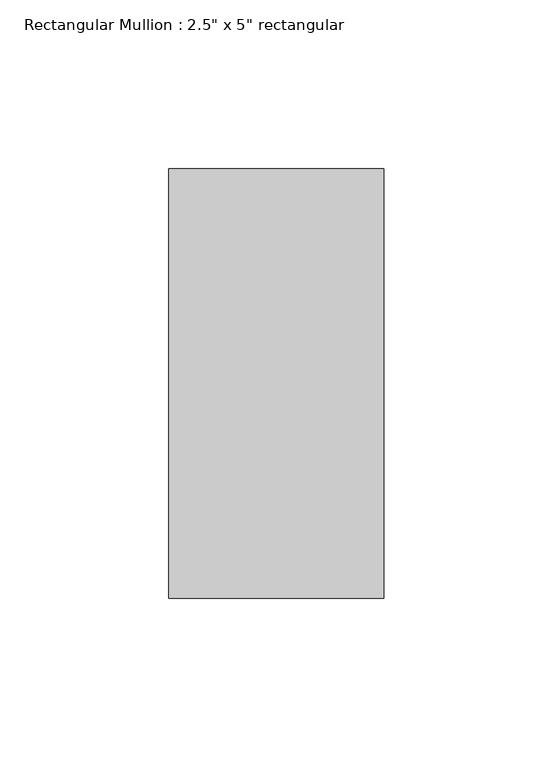
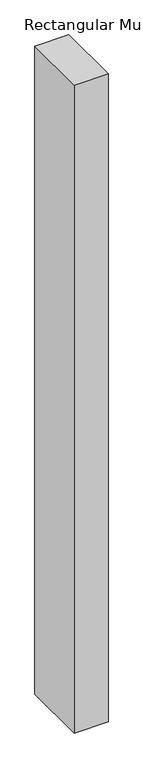
"""IFC4 building model written with IfcOpenShell, lengths in millimetres: member geometry."""

from ifc_helpers import new_model, si_unit, frame, origin, place, context, project, spatial, polyline, outline, extrude, source, transform, mapped, element, save


def member_cb331184(model_context):
    return source(origin(), model_context, "Body", "SweptSolid", [
        extrude(outline(polyline([(0.0, 63.5), (0.0, -63.5), (-63.5, -63.5), (-63.5, 63.5), (0.0, 63.5)])), frame((0.0, 0.0, -1281.4606784), z_axis=(0.0, 0.0, 1.0), x_axis=(1.0, 0.0, 0.0)), (0.0, 0.0, 1.0), 1281.4606784),
    ])


if __name__ == "__main__":
    model = new_model("IFC4")
    model_context = context("Model", 3, world=origin())
    ifc_project = project(units=[si_unit("LENGTHUNIT", "METRE", prefix="MILLI")], contexts=[model_context])
    site = spatial("IfcSite", under=ifc_project)
    building = spatial("IfcBuilding", under=site)
    placement = place(None, origin())
    member_shape = member_cb331184(model_context)
    element("IfcMember", 1, ObjectType="Rectangular Mullion : 2.5\" x 5\" rectangular", at=placement, inside=building, context=model_context, shape_type="MappedRepresentation", body=[
        mapped(member_shape, transform((0.0, 0.0, 0.0), x_axis=(1.0, 0.0, 0.0), y_axis=(0.0, 1.0, 0.0), z_axis=(0.0, 0.0, 1.0))),
    ])
    save(model, "model.ifc")

# Revit data of these elements
# Type "Rectangular Mullion : 2.5\" x 5\" rectangular"
#   built-in parameter 1007304 = 0.416667 (stored number, unit not read)
#   built-in parameter 1007301 = 0.104167 (stored number, unit not read)
#   built-in parameter 1007300 = 0.104167 (stored number, unit not read)
# Element 1 (IfcMember, "Rectangular Mullion : 2.5\" x 5\" rectangular")
#   Materials on its faces: "Aluminum"
# Materials
#   "Aluminum": class "Metal", colour RGB 247 247 247, transparency 0, Description = "Aluminum 6061", Cost = 0
